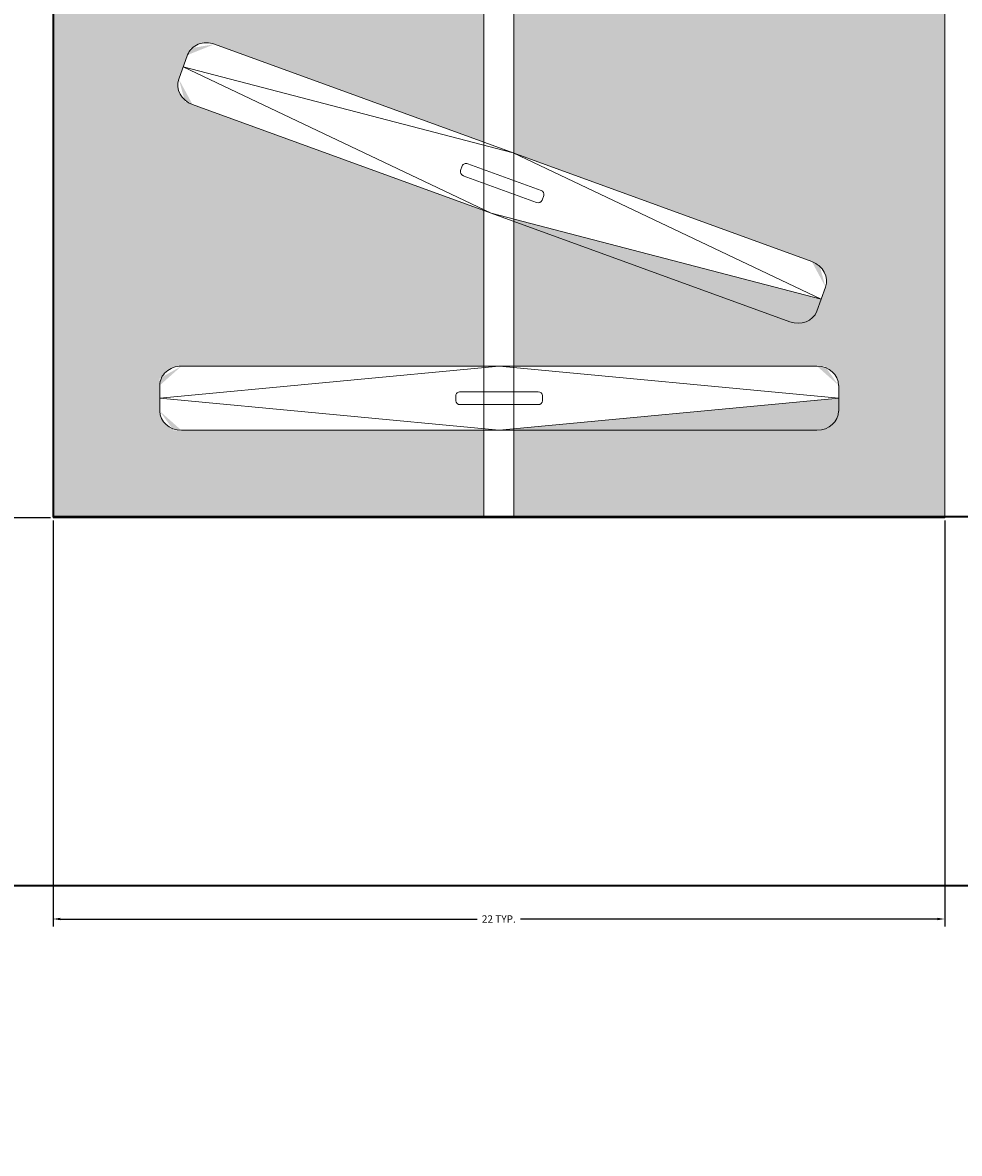
# Model space of a CAD drawing. Units: millimetres. Extents: x 27017497 to 27018854, y 7058029 to 7059154.
# Tile 64 of 91: x 27018319 to 27018342, y 7058126 to 7058154. Entities that reach past the tile are written whole.
import ezdxf

# ---------------------------------------------------------------- set-up
doc = ezdxf.new("R2010")
doc.units = ezdxf.units.MM
for name, color, linetype, lineweight in [('A-ANNO-DIMS', 2, 'Continuous', 18), ('A-FLOR-CASE', 8, 'Continuous', 20), ('A-FLOR-CASE-PATT', 44, 'Continuous', 13), ('A-WALL', 7, 'Continuous', 35)]:
    doc.layers.add(name, color=color, linetype=linetype, lineweight=lineweight)
doc.styles.get("Standard").update_dxf_attribs({"font": 'arial.ttf'})
doc.dimstyles.get("Standard").update_dxf_attribs({"dimtxt": 0.18, "dimasz": 0.18, "dimexe": 0.18, "dimexo": 0.0625, "dimgap": 0.09, "dimtad": 0, "dimtih": 1, "dimtoh": 1, "dimdec": 4, "dimzin": 0, "dimdsep": 46, "dimtxsty": 'Standard', "dimcen": 0.09, "dimadec": 0, "dimazin": 0, "dimtfac": 1, "dimtdec": 4, "dimtofl": 0, "dimtmove": 0, "dimatfit": 3, "dimfxl": 1, "dimtolj": 1, "dimtzin": 0, "dimarcsym": 0})

# ---------------------------------------------------------------- blocks, each defined once
blk = doc.blocks.new('WARDROBE-HANGING')
for p, q in [((0, 21.737), (65.212, 21.737)), ((65.212, 0), (65.212, 21.737)), ((62.293, 19.153), (61.511, 10.877)), ((62.606, 19.153), (61.98, 19.153)), ((62.293, 19.153), (63.076, 10.877)), ((60.171, 18.619), (59.582, 18.833)), ((58.961, 18.497), (53.661, 3.937)), ((59.877, 18.726), (56.311, 11.217)), ((59.877, 18.726), (57.782, 10.682)), ((61.511, 18.624), (61.511, 3.13)), ((63.076, 18.624), (63.076, 3.13)), ((60.431, 17.962), (55.132, 3.402)), ((57.224, 11.896), (56.574, 10.11)), ((57.466, 11.921), (57.349, 11.964)), ((62.356, 11.934), (62.231, 11.934)), ((57.519, 11.789), (56.868, 10.002)), ((62.137, 11.828), (62.137, 9.927)), ((62.45, 11.828), (62.45, 9.927)), ((0, 11.231), (65.212, 11.231)), ((54.216, 3.173), (56.311, 11.217)), ((62.293, 2.602), (61.511, 10.877)), ((62.293, 2.602), (63.076, 10.877)), ((0, 10.506), (65.212, 10.506)), ((54.216, 3.173), (57.782, 10.682)), ((56.744, 9.935), (56.626, 9.978)), ((62.356, 9.821), (62.231, 9.821)), ((54.51, 3.066), (53.922, 3.28)), ((62.606, 2.602), (61.98, 2.602)), ((0, 0), (65.212, 0))]:
    blk.add_line(p, q)
for centre, major_axis, start_param, end_param in [((61.98, 18.624), (0, 0.528), 0, 1.570796), ((62.606, 18.624), (0, 0.528), 4.712389, 6.283185), ((59.402, 18.336), (0.181, 0.496), 0, 1.570796), ((59.99, 18.122), (0.181, 0.496), -1.570796, 0), ((57.313, 11.864), (0.0361, 0.0993), 0, 1.570796), ((57.43, 11.821), (0.0361, 0.0993), 4.712389, 6.283185), ((62.231, 11.828), (0, 0.106), 0, 1.570796), ((62.356, 11.828), (0, 0.106), -1.570796, 0), ((56.662, 10.077), (0.0361, 0.0993), 1.570796, 3.141593), ((56.78, 10.035), (0.0361, 0.0993), 3.141593, 4.712389), ((62.231, 9.927), (0, 0.106), 1.570796, 3.141593), ((62.356, 9.927), (0, 0.106), 3.141593, 4.712389), ((54.102, 3.777), (0.181, 0.496), 1.570796, 3.141593), ((54.691, 3.562), (0.181, 0.496), 3.141593, 4.712389), ((61.98, 3.13), (0, 0.528), 1.570796, 3.141593), ((62.606, 3.13), (0, 0.528), 3.141593, 4.712389)]:
    blk.add_ellipse(centre, major_axis=major_axis, ratio=0.888892, start_param=start_param, end_param=end_param)
blk = doc.blocks.new('*D33')
at = {"layer": 'A-ANNO-DIMS', "color": 0, "lineweight": -2, "transparency": 16777216}
for p, q in [((27018319.543, 7058207.1), (27018309.644, 7058207.1)), ((27018309.824, 7058206.92), (27018309.824, 7058174.677)), ((27018309.824, 7058142.068), (27018309.824, 7058174.311)), ((27018319.543, 7058141.888), (27018309.644, 7058141.888))]:
    blk.add_line(p, q, dxfattribs=at)
at = {"layer": 'A-ANNO-DIMS', "color": 0, "transparency": 16777216}
for points in [[(27018309.794, 7058206.92), (27018309.854, 7058206.92), (27018309.824, 7058207.1)], [(27018309.794, 7058142.068), (27018309.854, 7058142.068), (27018309.824, 7058141.888)]]:
    blk.add_solid(points, dxfattribs=at)
at = {"layer": 'Defpoints', "color": 0, "transparency": 16777216}
for p in [(27018319.606, 7058207.1), (27018309.824, 7058141.888), (27018319.606, 7058141.888)]:
    blk.add_point(p, dxfattribs=at)
at = {"layer": 'A-ANNO-DIMS', "color": 0, "transparency": 16777216, "insert": (27018309.824, 7058174.494), "char_height": 0.18, "attachment_point": 5}
blk.add_mtext('\\A1;WARDROBE 65 TYP.', dxfattribs=at)
blk = doc.blocks.new('*D34')
at = {"layer": 'A-ANNO-DIMS', "color": 0, "lineweight": -2, "transparency": 16777216}
for p, q in [((27018319.606, 7058141.826), (27018319.606, 7058131.926)), ((27018341.343, 7058141.826), (27018341.343, 7058131.926)), ((27018319.786, 7058132.106), (27018329.945, 7058132.106)), ((27018341.163, 7058132.106), (27018331.004, 7058132.106))]:
    blk.add_line(p, q, dxfattribs=at)
at = {"layer": 'A-ANNO-DIMS', "color": 0, "transparency": 16777216}
for points in [[(27018319.786, 7058132.136), (27018319.786, 7058132.076), (27018319.606, 7058132.106)], [(27018341.163, 7058132.136), (27018341.163, 7058132.076), (27018341.343, 7058132.106)]]:
    blk.add_solid(points, dxfattribs=at)
at = {"layer": 'Defpoints', "color": 0, "transparency": 16777216}
for p in [(27018319.606, 7058141.888), (27018341.343, 7058141.888), (27018341.343, 7058132.106)]:
    blk.add_point(p, dxfattribs=at)
at = {"layer": 'A-ANNO-DIMS', "color": 0, "transparency": 16777216, "insert": (27018330.474, 7058132.106), "char_height": 0.18, "attachment_point": 5}
blk.add_mtext('\\A1;22 TYP.', dxfattribs=at)
blk = doc.blocks.new('*D47')
at = {"layer": 'A-ANNO-DIMS', "color": 0, "lineweight": -2, "transparency": 16777216}
for p, q in [((27017561.166, 7058294.35), (27017561.166, 7058028.6)), ((27018790.606, 7058294.35), (27018790.606, 7058028.6)), ((27017561.346, 7058028.78), (27018175.431, 7058028.78)), ((27018790.426, 7058028.78), (27018176.341, 7058028.78))]:
    blk.add_line(p, q, dxfattribs=at)
at = {"layer": 'A-ANNO-DIMS', "color": 0, "transparency": 16777216}
for points in [[(27017561.346, 7058028.81), (27017561.346, 7058028.75), (27017561.166, 7058028.78)], [(27018790.426, 7058028.81), (27018790.426, 7058028.75), (27018790.606, 7058028.78)]]:
    blk.add_solid(points, dxfattribs=at)
at = {"layer": 'Defpoints', "color": 0, "transparency": 16777216}
for p in [(27017561.166, 7058294.412), (27018790.606, 7058294.412), (27018790.606, 7058028.78)]:
    blk.add_point(p, dxfattribs=at)
at = {"layer": 'A-ANNO-DIMS', "color": 0, "transparency": 16777216, "insert": (27018175.886, 7058028.78), "char_height": 0.18, "attachment_point": 5}
blk.add_mtext('\\A1;1229.4', dxfattribs=at)
blk = doc.blocks.new('*D48')
at = {"layer": 'A-ANNO-DIMS', "color": 0, "lineweight": -2, "transparency": 16777216}
for p, q in [((27018463.498, 7058622.912), (27017497.536, 7058622.912)), ((27017497.716, 7058622.732), (27017497.716, 7058357.753)), ((27017497.716, 7058092.41), (27017497.716, 7058357.389)), ((27018555.129, 7058092.23), (27017497.536, 7058092.23))]:
    blk.add_line(p, q, dxfattribs=at)
at = {"layer": 'A-ANNO-DIMS', "color": 0, "transparency": 16777216}
for points in [[(27017497.686, 7058622.732), (27017497.746, 7058622.732), (27017497.716, 7058622.912)], [(27017497.686, 7058092.41), (27017497.746, 7058092.41), (27017497.716, 7058092.23)]]:
    blk.add_solid(points, dxfattribs=at)
at = {"layer": 'Defpoints', "color": 0, "transparency": 16777216}
for p in [(27018463.561, 7058622.912), (27017497.716, 7058092.23), (27018555.192, 7058092.23)]:
    blk.add_point(p, dxfattribs=at)
at = {"layer": 'A-ANNO-DIMS', "color": 0, "transparency": 16777216, "insert": (27017497.716, 7058357.571), "char_height": 0.18, "attachment_point": 5}
blk.add_mtext('\\A1;530.7', dxfattribs=at)

msp = doc.modelspace()

# ---------------------------------------------------------------- hatches: boundary and pattern name
at = {"layer": 'A-FLOR-CASE-PATT'}
h = msp.add_hatch(color=256, dxfattribs=at)
h.dxf.hatch_style = 1
edge = h.paths.add_edge_path()
edge.add_line((27018341.343, 7058207.055), (27018330.837, 7058207.055))
edge.add_line((27018330.837, 7058207.055), (27018330.837, 7058203.02))
edge.add_line((27018330.837, 7058203.02), (27018338.424, 7058203.02))
edge.add_ellipse((27018338.23, 7058202.551), major_axis=(0.528, 0), ratio=0.888892, start_angle=0, end_angle=90, ccw=False)
edge.add_line((27018338.758, 7058202.551), (27018338.758, 7058202.238))
edge.add_line((27018338.758, 7058202.238), (27018330.837, 7058201.488))
edge.add_line((27018330.837, 7058201.488), (27018330.837, 7058199.747))
edge.add_line((27018330.837, 7058199.747), (27018338.424, 7058199.747))
edge.add_ellipse((27018338.23, 7058199.277), major_axis=(0.528, 0), ratio=0.888892, start_angle=0, end_angle=90, ccw=False)
edge.add_line((27018338.758, 7058199.277), (27018338.758, 7058198.964))
edge.add_line((27018338.758, 7058198.964), (27018330.837, 7058198.215))
edge.add_line((27018330.837, 7058198.215), (27018330.837, 7058193.415))
edge.add_line((27018330.837, 7058193.415), (27018338.284, 7058190.704))
edge.add_ellipse((27018337.942, 7058190.329), major_axis=(0.496, -0.181), ratio=0.888892, start_angle=0, end_angle=90, ccw=False)
edge.add_line((27018338.439, 7058190.148), (27018338.331, 7058189.854))
edge.add_line((27018338.331, 7058189.854), (27018330.837, 7058191.806))
edge.add_line((27018330.837, 7058191.806), (27018330.837, 7058188.22))
edge.add_line((27018330.837, 7058188.22), (27018338.424, 7058188.22))
edge.add_ellipse((27018338.23, 7058187.75), major_axis=(0.528, 0), ratio=0.888892, start_angle=0, end_angle=90, ccw=False)
edge.add_line((27018338.758, 7058187.75), (27018338.758, 7058187.437))
edge.add_line((27018338.758, 7058187.437), (27018330.837, 7058186.688))
edge.add_line((27018330.837, 7058186.688), (27018330.837, 7058181.982))
edge.add_line((27018330.837, 7058181.982), (27018338.424, 7058181.982))
edge.add_ellipse((27018338.23, 7058181.513), major_axis=(0.528, 0), ratio=0.888892, start_angle=0, end_angle=90, ccw=False)
edge.add_line((27018338.758, 7058181.513), (27018338.758, 7058181.199))
edge.add_line((27018338.758, 7058181.199), (27018330.837, 7058180.45))
edge.add_line((27018330.837, 7058180.45), (27018330.837, 7058178.709))
edge.add_line((27018330.837, 7058178.709), (27018338.424, 7058178.709))
edge.add_ellipse((27018338.23, 7058178.239), major_axis=(0.528, 0), ratio=0.888892, start_angle=0, end_angle=90, ccw=False)
edge.add_line((27018338.758, 7058178.239), (27018338.758, 7058177.926))
edge.add_line((27018338.758, 7058177.926), (27018330.837, 7058177.177))
edge.add_line((27018330.837, 7058177.177), (27018330.837, 7058173.878))
edge.add_line((27018330.837, 7058173.878), (27018338.284, 7058171.167))
edge.add_ellipse((27018337.942, 7058170.792), major_axis=(0.496, -0.181), ratio=0.888892, start_angle=0, end_angle=90, ccw=False)
edge.add_line((27018338.439, 7058170.611), (27018338.331, 7058170.317))
edge.add_line((27018338.331, 7058170.317), (27018330.837, 7058172.269))
edge.add_line((27018330.837, 7058172.269), (27018330.837, 7058168.293))
edge.add_line((27018330.837, 7058168.293), (27018338.424, 7058168.293))
edge.add_ellipse((27018338.23, 7058167.824), major_axis=(0.528, 0), ratio=0.888892, start_angle=0, end_angle=90, ccw=False)
edge.add_line((27018338.758, 7058167.824), (27018338.758, 7058167.511))
edge.add_line((27018338.758, 7058167.511), (27018330.837, 7058166.762))
edge.add_line((27018330.837, 7058166.762), (27018330.837, 7058160.389))
edge.add_line((27018330.837, 7058160.389), (27018338.424, 7058160.389))
edge.add_ellipse((27018338.23, 7058159.92), major_axis=(0.528, 0), ratio=0.888892, start_angle=0, end_angle=90, ccw=False)
edge.add_line((27018338.758, 7058159.92), (27018338.758, 7058159.607))
edge.add_line((27018338.758, 7058159.607), (27018330.837, 7058158.858))
edge.add_line((27018330.837, 7058158.858), (27018330.837, 7058157.116))
edge.add_line((27018330.837, 7058157.116), (27018338.424, 7058157.116))
edge.add_ellipse((27018338.23, 7058156.647), major_axis=(0.528, 0), ratio=0.888892, start_angle=0, end_angle=90, ccw=False)
edge.add_line((27018338.758, 7058156.647), (27018338.758, 7058156.334))
edge.add_line((27018338.758, 7058156.334), (27018330.837, 7058155.585))
edge.add_line((27018330.837, 7058155.585), (27018330.837, 7058150.784))
edge.add_line((27018330.837, 7058150.784), (27018338.284, 7058148.073))
edge.add_ellipse((27018337.942, 7058147.698), major_axis=(0.496, -0.181), ratio=0.888892, start_angle=0, end_angle=90, ccw=False)
edge.add_line((27018338.439, 7058147.517), (27018338.331, 7058147.223))
edge.add_line((27018338.331, 7058147.223), (27018330.837, 7058149.175))
edge.add_line((27018330.837, 7058149.175), (27018330.837, 7058145.589))
edge.add_line((27018330.837, 7058145.589), (27018338.424, 7058145.589))
edge.add_ellipse((27018338.23, 7058145.119), major_axis=(0.528, 0), ratio=0.888892, start_angle=0, end_angle=90, ccw=False)
edge.add_line((27018338.758, 7058145.119), (27018338.758, 7058144.806))
edge.add_line((27018338.758, 7058144.806), (27018330.837, 7058144.057))
edge.add_line((27018330.837, 7058144.057), (27018330.837, 7058141.912))
edge.add_line((27018330.837, 7058141.912), (27018341.343, 7058141.912))
edge.add_line((27018341.343, 7058141.912), (27018341.343, 7058207.055))
edge = h.paths.add_edge_path()
edge.add_line((27018330.112, 7058207.055), (27018319.606, 7058207.055))
edge.add_line((27018319.606, 7058207.055), (27018319.606, 7058141.912))
edge.add_line((27018319.606, 7058141.912), (27018330.112, 7058141.912))
edge.add_line((27018330.112, 7058141.912), (27018330.112, 7058144.024))
edge.add_line((27018330.112, 7058144.024), (27018322.543, 7058144.024))
edge.add_ellipse((27018322.736, 7058144.493), major_axis=(0.528, 0), ratio=0.888892, start_angle=180, end_angle=270, ccw=False)
edge.add_line((27018322.208, 7058144.493), (27018322.208, 7058145.291))
edge.add_ellipse((27018322.736, 7058145.119), major_axis=(0.528, 0), ratio=0.888892, start_angle=90, end_angle=180, ccw=False)
edge.add_line((27018322.736, 7058145.589), (27018330.112, 7058145.589))
edge.add_line((27018330.112, 7058145.589), (27018330.112, 7058149.382))
edge.add_line((27018330.112, 7058149.382), (27018322.826, 7058152.034))
edge.add_ellipse((27018323.168, 7058152.409), major_axis=(0.496, -0.181), ratio=0.888892, start_angle=180, end_angle=270, ccw=False)
edge.add_line((27018322.672, 7058152.59), (27018322.945, 7058153.34))
edge.add_ellipse((27018323.382, 7058152.997), major_axis=(0.496, -0.181), ratio=0.888892, start_angle=90, end_angle=180, ccw=False)
edge.add_line((27018323.543, 7058153.439), (27018330.112, 7058151.048))
edge.add_line((27018330.112, 7058151.048), (27018330.112, 7058155.551))
edge.add_line((27018330.112, 7058155.551), (27018322.543, 7058155.551))
edge.add_ellipse((27018322.736, 7058156.021), major_axis=(0.528, 0), ratio=0.888892, start_angle=180, end_angle=270, ccw=False)
edge.add_line((27018322.208, 7058156.021), (27018322.208, 7058156.819))
edge.add_ellipse((27018322.736, 7058156.647), major_axis=(0.528, 0), ratio=0.888892, start_angle=90, end_angle=180, ccw=False)
edge.add_line((27018322.736, 7058157.116), (27018330.112, 7058157.116))
edge.add_line((27018330.112, 7058157.116), (27018330.112, 7058158.824))
edge.add_line((27018330.112, 7058158.824), (27018322.543, 7058158.824))
edge.add_ellipse((27018322.736, 7058159.294), major_axis=(0.528, 0), ratio=0.888892, start_angle=180, end_angle=270, ccw=False)
edge.add_line((27018322.208, 7058159.294), (27018322.208, 7058160.092))
edge.add_ellipse((27018322.736, 7058159.92), major_axis=(0.528, 0), ratio=0.888892, start_angle=90, end_angle=180, ccw=False)
edge.add_line((27018322.736, 7058160.389), (27018330.112, 7058160.389))
edge.add_line((27018330.112, 7058160.389), (27018330.112, 7058166.728))
edge.add_line((27018330.112, 7058166.728), (27018322.543, 7058166.728))
edge.add_ellipse((27018322.736, 7058167.198), major_axis=(0.528, 0), ratio=0.888892, start_angle=180, end_angle=270, ccw=False)
edge.add_line((27018322.208, 7058167.198), (27018322.208, 7058167.996))
edge.add_ellipse((27018322.736, 7058167.824), major_axis=(0.528, 0), ratio=0.888892, start_angle=90, end_angle=180, ccw=False)
edge.add_line((27018322.736, 7058168.293), (27018330.112, 7058168.293))
edge.add_line((27018330.112, 7058168.293), (27018330.112, 7058172.476))
edge.add_line((27018330.112, 7058172.476), (27018322.826, 7058175.128))
edge.add_ellipse((27018323.168, 7058175.503), major_axis=(0.496, -0.181), ratio=0.888892, start_angle=180, end_angle=270, ccw=False)
edge.add_line((27018322.672, 7058175.684), (27018322.945, 7058176.433))
edge.add_ellipse((27018323.382, 7058176.091), major_axis=(0.496, -0.181), ratio=0.888892, start_angle=90, end_angle=180, ccw=False)
edge.add_line((27018323.543, 7058176.533), (27018330.112, 7058174.142))
edge.add_line((27018330.112, 7058174.142), (27018330.112, 7058177.144))
edge.add_line((27018330.112, 7058177.144), (27018322.543, 7058177.144))
edge.add_ellipse((27018322.736, 7058177.613), major_axis=(0.528, 0), ratio=0.888892, start_angle=180, end_angle=270, ccw=False)
edge.add_line((27018322.208, 7058177.613), (27018322.208, 7058178.411))
edge.add_ellipse((27018322.736, 7058178.239), major_axis=(0.528, 0), ratio=0.888892, start_angle=90, end_angle=180, ccw=False)
edge.add_line((27018322.736, 7058178.709), (27018330.112, 7058178.709))
edge.add_line((27018330.112, 7058178.709), (27018330.112, 7058180.417))
edge.add_line((27018330.112, 7058180.417), (27018322.543, 7058180.417))
edge.add_ellipse((27018322.736, 7058180.886), major_axis=(0.528, 0), ratio=0.888892, start_angle=180, end_angle=270, ccw=False)
edge.add_line((27018322.208, 7058180.886), (27018322.208, 7058181.684))
edge.add_ellipse((27018322.736, 7058181.513), major_axis=(0.528, 0), ratio=0.888892, start_angle=90, end_angle=180, ccw=False)
edge.add_line((27018322.736, 7058181.982), (27018330.112, 7058181.982))
edge.add_line((27018330.112, 7058181.982), (27018330.112, 7058186.655))
edge.add_line((27018330.112, 7058186.655), (27018322.543, 7058186.655))
edge.add_ellipse((27018322.736, 7058187.124), major_axis=(0.528, 0), ratio=0.888892, start_angle=180, end_angle=270, ccw=False)
edge.add_line((27018322.208, 7058187.124), (27018322.208, 7058187.922))
edge.add_ellipse((27018322.736, 7058187.75), major_axis=(0.528, 0), ratio=0.888892, start_angle=90, end_angle=180, ccw=False)
edge.add_line((27018322.736, 7058188.22), (27018330.112, 7058188.22))
edge.add_line((27018330.112, 7058188.22), (27018330.112, 7058192.013))
edge.add_line((27018330.112, 7058192.013), (27018322.826, 7058194.665))
edge.add_ellipse((27018323.168, 7058195.04), major_axis=(0.496, -0.181), ratio=0.888892, start_angle=180, end_angle=270, ccw=False)
edge.add_line((27018322.672, 7058195.22), (27018322.945, 7058195.97))
edge.add_ellipse((27018323.382, 7058195.628), major_axis=(0.496, -0.181), ratio=0.888892, start_angle=90, end_angle=180, ccw=False)
edge.add_line((27018323.543, 7058196.069), (27018330.112, 7058193.678))
edge.add_line((27018330.112, 7058193.678), (27018330.112, 7058198.182))
edge.add_line((27018330.112, 7058198.182), (27018322.543, 7058198.182))
edge.add_ellipse((27018322.736, 7058198.651), major_axis=(0.528, 0), ratio=0.888892, start_angle=180, end_angle=270, ccw=False)
edge.add_line((27018322.208, 7058198.651), (27018322.208, 7058199.449))
edge.add_ellipse((27018322.736, 7058199.277), major_axis=(0.528, 0), ratio=0.888892, start_angle=90, end_angle=180, ccw=False)
edge.add_line((27018322.736, 7058199.747), (27018330.112, 7058199.747))
edge.add_line((27018330.112, 7058199.747), (27018330.112, 7058201.455))
edge.add_line((27018330.112, 7058201.455), (27018322.543, 7058201.455))
edge.add_ellipse((27018322.736, 7058201.924), major_axis=(0.528, 0), ratio=0.888892, start_angle=180, end_angle=270, ccw=False)
edge.add_line((27018322.208, 7058201.924), (27018322.208, 7058202.722))
edge.add_ellipse((27018322.736, 7058202.551), major_axis=(0.528, 0), ratio=0.888892, start_angle=90, end_angle=180, ccw=False)
edge.add_line((27018322.736, 7058203.02), (27018330.112, 7058203.02))
edge.add_line((27018330.112, 7058203.02), (27018330.112, 7058207.055))
h.paths.add_polyline_path([(27018341.31, 7058294.412), (27018319.606, 7058294.412), (27018319.606, 7058207.1), (27018341.31, 7058207.1)])
h.paths.add_polyline_path([(27018354.358, 7058255.592), (27018354.358, 7058256.057, -0.414214), (27018354.869, 7058256.569), (27018346.477, 7058256.569, -0.414214), (27018345.197, 7058257.848), (27018345.197, 7058259.128, -0.414214), (27018346.477, 7058260.407), (27018343.868, 7058260.407, 0.290979), (27018341.551, 7058258.934), (27018341.551, 7058242.534, 0.290979), (27018343.868, 7058241.06), (27018346.477, 7058241.06, -0.414214), (27018345.197, 7058242.34), (27018345.197, 7058243.619, -0.414214), (27018346.477, 7058244.899), (27018353.078, 7058244.899, 0.414214), (27018354.358, 7058246.178)])
h.paths.add_polyline_path([(27018356.917, 7058260.407), (27018346.477, 7058260.407, 0.414214), (27018345.197, 7058259.128), (27018345.197, 7058257.848, 0.414214), (27018346.477, 7058256.569), (27018355.637, 7058256.569), (27018355.637, 7058244.899), (27018346.477, 7058244.899, 0.414214), (27018345.197, 7058243.619), (27018345.197, 7058242.34, 0.414214), (27018346.477, 7058241.06), (27018356.917, 7058241.06, 0.414214), (27018359.476, 7058243.619), (27018359.476, 7058257.848, 0.414214)])
h.paths.add_polyline_path([(27018355.637, 7058252.362), (27018355.637, 7058256.057, 0.490314), (27018354.997, 7058256.553, 0.490314), (27018354.358, 7058256.057), (27018354.358, 7058255.592), (27018354.358, 7058245.411, 0.490314), (27018354.997, 7058244.915, 0.490314), (27018355.637, 7058245.411)], flags=17)

# ---------------------------------------------------------------- linework, layer by layer
at = {"layer": 'A-WALL'}
for p, q in [((27018319.606, 7058386.803), (27018319.606, 7058141.912)), ((27018468.106, 7058141.912), (27018319.606, 7058141.912)), ((27018468.106, 7058132.912), (27018310.606, 7058132.912))]:
    msp.add_line(p, q, dxfattribs=at)

# ---------------------------------------------------------------- block references
at = {"layer": 'A-FLOR-CASE', "rotation": 270}
msp.add_blockref('WARDROBE-HANGING', (27018319.606, 7058207.1), dxfattribs=at)

# ---------------------------------------------------------------- dimensions: what is measured, and where the dimension line sits
at = {"layer": 'A-ANNO-DIMS'}
dim = msp.add_linear_dim(base=(27017497.716, 7058092.23), p1=(27018463.561, 7058622.912), p2=(27018555.192, 7058092.23), angle=90, dimstyle='Standard', override={"dimdec": 1, "dimlfac": 1, "dimrnd": 0, "dimzin": 0, "dimdsep": 46, "dimlunit": 2}, dxfattribs=at)
dim.commit()
dim.dimension.update_dxf_attribs({"geometry": '*D48', "text_midpoint": (27017497.716, 7058357.571)})
dim = msp.add_linear_dim(base=(27018790.606, 7058028.78), p1=(27017561.166, 7058294.412), p2=(27018790.606, 7058294.412), dimstyle='Standard', override={"dimdec": 1, "dimlfac": 1, "dimrnd": 0, "dimzin": 0, "dimdsep": 46, "dimlunit": 2}, dxfattribs=at)
dim.commit()
dim.dimension.update_dxf_attribs({"geometry": '*D47', "text_midpoint": (27018175.886, 7058028.78)})
dim = msp.add_linear_dim(base=(27018309.824, 7058141.888), p1=(27018319.606, 7058207.1), p2=(27018319.606, 7058141.888), angle=270, text='WARDROBE <> TYP.', dimstyle='Standard', override={"dimdec": 0, "dimlfac": 1, "dimrnd": 0, "dimzin": 0, "dimdsep": 46, "dimlunit": 2}, dxfattribs=at)
dim.commit()
dim.dimension.update_dxf_attribs({"geometry": '*D33', "text_midpoint": (27018309.824, 7058174.494)})
dim = msp.add_linear_dim(base=(27018341.343, 7058132.106), p1=(27018319.606, 7058141.888), p2=(27018341.343, 7058141.888), text='<> TYP.', dimstyle='Standard', override={"dimdec": 0, "dimlfac": 1, "dimrnd": 0, "dimzin": 0, "dimdsep": 46, "dimlunit": 2}, dxfattribs=at)
dim.commit()
dim.dimension.update_dxf_attribs({"geometry": '*D34', "text_midpoint": (27018330.474, 7058132.106)})

doc.saveas('drawing.dxf')
